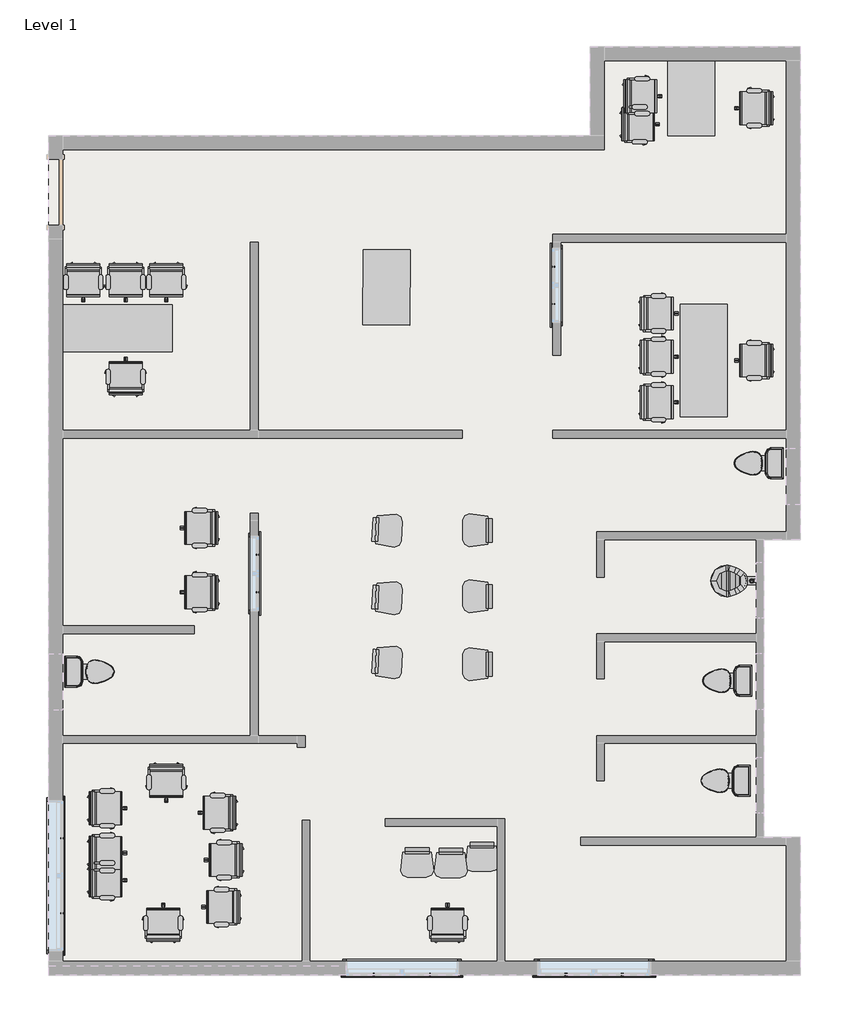
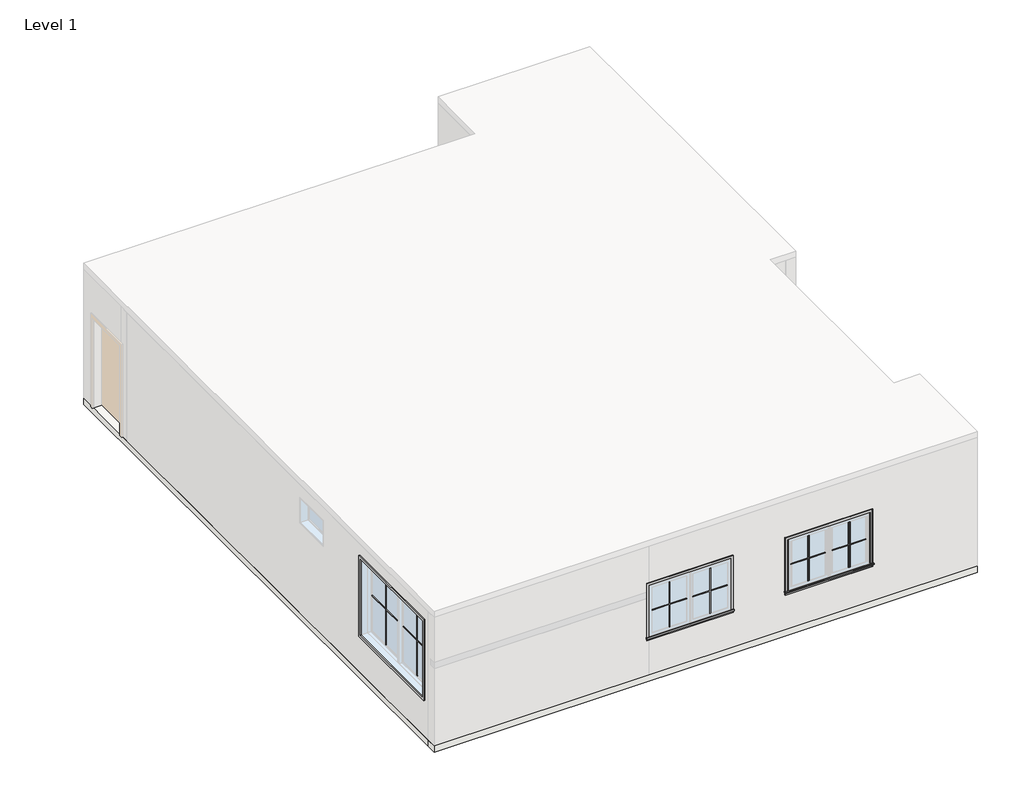
# One storey, part 2 of 2: 35 furniture elements, 28 proxies, 5 flow terminals, 2 slabs.
"""IFC4 building model written with IfcOpenShell, lengths in millimetres."""

from ifc_helpers import new_model, si_unit, frame, origin, place, context, project, spatial, polyline, outline, extrude, transform, mapped, element, save
from components import muntin_pattern_2x2_muntin_pattern_2x2_dc2504c2, muntin_pattern_2x2_muntin_pattern_2x2_0aa094e9, muntin_pattern_2x2_muntin_pattern_2x2_bb8d4d84, muntin_pattern_2x2_muntin_pattern_2x2_d03a1f3c, muntin_pattern_2x2_muntin_pattern_2x2_2b4d9f72, muntin_pattern_2x2_muntin_pattern_2x2_ef995ed3, trim_window_exterior_flat_with_sill_db7a9870, trim_window_exterior_flat_with_sill_02d88a07, trim_window_exterior_flat_with_sill_359ed2ce, trim_window_exterior_flat_with_sill_b7e4d11c, trim_window_interior_flat_picture_frame_bbff334a, trim_window_interior_flat_picture_frame_03e64d7c, trim_window_interior_flat_picture_frame_939a8053, trim_window_interior_flat_picture_frame_936b8d2a, flow_terminal_a02a0911, toilet_domestic_3d_toilet_domestic_3d_ba6479b0, toilet_domestic_3d_toilet_domestic_3d_30431060, chair_desk_chair_desk_7ad88740, chair_task_arms_chair_task_arms_bb362225, chair_task_arms_chair_task_arms_83a3c27c, furniture_acc2807d, furniture_03292632, furniture_fc20a73e, furniture_102a29e2

model = new_model("IFC4")

# Units and contexts
model_context = context("Model", 3, world=origin())
ifc_project = project(units=[si_unit("LENGTHUNIT", "METRE", prefix="MILLI")], contexts=[model_context])

# Site, building, storey
site = spatial("IfcSite", under=ifc_project)
building = spatial("IfcBuilding", under=site)
storey = spatial("IfcBuildingStorey", under=building, Name="Level 1", Elevation=0.0)

# Proxies
placement = place(None, origin())
muntin_pattern_2x2_muntin_pattern_2x2_shape = muntin_pattern_2x2_muntin_pattern_2x2_dc2504c2(model_context)
element("IfcBuildingElementProxy", 1, Name="Muntin Pattern_2x2 : Muntin Pattern_2x2", ObjectType="Muntin Pattern_2x2 : Muntin Pattern_2x2", at=placement, inside=storey, context=model_context, shape_type="MappedRepresentation", body=[
    mapped(muntin_pattern_2x2_muntin_pattern_2x2_shape, transform((-1125.8570713, -5476.875, 984.25), x_axis=(-1.0, 0.0, 0.0), y_axis=(0.0, -1.0, 0.0), z_axis=(0.0, 0.0, 1.0))),
])
element("IfcBuildingElementProxy", 2, Name="Muntin Pattern_2x2 : Muntin Pattern_2x2", ObjectType="Muntin Pattern_2x2 : Muntin Pattern_2x2", at=placement, inside=storey, context=model_context, shape_type="MappedRepresentation", body=[
    mapped(muntin_pattern_2x2_muntin_pattern_2x2_shape, transform((1979.6125, -5476.875, 984.25), x_axis=(-1.0, 0.0, 0.0), y_axis=(0.0, -1.0, 0.0), z_axis=(0.0, 0.0, 1.0))),
])
element("IfcBuildingElementProxy", 3, Name="Muntin Pattern_2x2 : Muntin Pattern_2x2", ObjectType="Muntin Pattern_2x2 : Muntin Pattern_2x2", at=placement, inside=storey, context=model_context, shape_type="MappedRepresentation", body=[
    mapped(muntin_pattern_2x2_muntin_pattern_2x2_shape, transform((2005.0125, -5476.875, 984.25), x_axis=(-1.0, 0.0, 0.0), y_axis=(0.0, -1.0, 0.0), z_axis=(0.0, 0.0, 1.0))),
])
muntin_pattern_2x2_muntin_pattern_2x2_2_shape = muntin_pattern_2x2_muntin_pattern_2x2_0aa094e9(model_context)
element("IfcBuildingElementProxy", 4, Name="Muntin Pattern_2x2 : Muntin Pattern_2x2", ObjectType="Muntin Pattern_2x2 : Muntin Pattern_2x2", at=placement, inside=storey, context=model_context, shape_type="MappedRepresentation", body=[
    mapped(muntin_pattern_2x2_muntin_pattern_2x2_2_shape, transform((-2037.0820713, -5476.875, 984.25), x_axis=(1.0, 0.0, 0.0), y_axis=(0.0, 1.0, 0.0), z_axis=(0.0, 0.0, 1.0))),
])
element("IfcBuildingElementProxy", 5, Name="Muntin Pattern_2x2 : Muntin Pattern_2x2", ObjectType="Muntin Pattern_2x2 : Muntin Pattern_2x2", at=placement, inside=storey, context=model_context, shape_type="MappedRepresentation", body=[
    mapped(muntin_pattern_2x2_muntin_pattern_2x2_2_shape, transform((1068.3875, -5476.875, 984.25), x_axis=(1.0, 0.0, 0.0), y_axis=(0.0, 1.0, 0.0), z_axis=(0.0, 0.0, 1.0))),
])
element("IfcBuildingElementProxy", 6, Name="Muntin Pattern_2x2 : Muntin Pattern_2x2", ObjectType="Muntin Pattern_2x2 : Muntin Pattern_2x2", at=placement, inside=storey, context=model_context, shape_type="MappedRepresentation", body=[
    mapped(muntin_pattern_2x2_muntin_pattern_2x2_2_shape, transform((1093.7875, -5476.875, 984.25), x_axis=(1.0, 0.0, 0.0), y_axis=(0.0, 1.0, 0.0), z_axis=(0.0, 0.0, 1.0))),
])
muntin_pattern_2x2_muntin_pattern_2x2_3_shape = muntin_pattern_2x2_muntin_pattern_2x2_bb8d4d84(model_context)
element("IfcBuildingElementProxy", 7, Name="Muntin Pattern_2x2 : Muntin Pattern_2x2", ObjectType="Muntin Pattern_2x2 : Muntin Pattern_2x2", at=placement, inside=storey, context=model_context, shape_type="MappedRepresentation", body=[
    mapped(muntin_pattern_2x2_muntin_pattern_2x2_3_shape, transform((-7096.125, -3265.4875, 984.25), x_axis=(0.0, -1.0, 0.0), y_axis=(1.0, 0.0, 0.0), z_axis=(0.0, 0.0, 1.0))),
])
muntin_pattern_2x2_muntin_pattern_2x2_4_shape = muntin_pattern_2x2_muntin_pattern_2x2_d03a1f3c(model_context)
element("IfcBuildingElementProxy", 8, Name="Muntin Pattern_2x2 : Muntin Pattern_2x2", ObjectType="Muntin Pattern_2x2 : Muntin Pattern_2x2", at=placement, inside=storey, context=model_context, shape_type="MappedRepresentation", body=[
    mapped(muntin_pattern_2x2_muntin_pattern_2x2_4_shape, transform((-7096.125, -4481.5125, 984.25), x_axis=(0.0, 1.0, 0.0), y_axis=(-1.0, 0.0, 0.0), z_axis=(0.0, 0.0, 1.0))),
])
muntin_pattern_2x2_muntin_pattern_2x2_5_shape = muntin_pattern_2x2_muntin_pattern_2x2_2b4d9f72(model_context)
element("IfcBuildingElementProxy", 9, Name="Muntin Pattern_2x2 : Muntin Pattern_2x2", ObjectType="Muntin Pattern_2x2 : Muntin Pattern_2x2", at=placement, inside=storey, context=model_context, shape_type="MappedRepresentation", body=[
    mapped(muntin_pattern_2x2_muntin_pattern_2x2_5_shape, transform((-3921.125, 1332.4236463, 984.25), x_axis=(0.0, -1.0, 0.0), y_axis=(1.0, 0.0, 0.0), z_axis=(0.0, 0.0, 1.0))),
])
element("IfcBuildingElementProxy", 10, Name="Muntin Pattern_2x2 : Muntin Pattern_2x2", ObjectType="Muntin Pattern_2x2 : Muntin Pattern_2x2", at=placement, inside=storey, context=model_context, shape_type="MappedRepresentation", body=[
    mapped(muntin_pattern_2x2_muntin_pattern_2x2_5_shape, transform((-3921.125, 1332.4236463, 984.25), x_axis=(0.0, -1.0, 0.0), y_axis=(1.0, 0.0, 0.0), z_axis=(0.0, 0.0, 1.0))),
])
element("IfcBuildingElementProxy", 11, Name="Muntin Pattern_2x2 : Muntin Pattern_2x2", ObjectType="Muntin Pattern_2x2 : Muntin Pattern_2x2", at=placement, inside=storey, context=model_context, shape_type="MappedRepresentation", body=[
    mapped(muntin_pattern_2x2_muntin_pattern_2x2_5_shape, transform((873.125, 5399.0875, 984.25), x_axis=(0.0, 1.0, 0.0), y_axis=(-1.0, 0.0, 0.0), z_axis=(0.0, 0.0, 1.0))),
])
muntin_pattern_2x2_muntin_pattern_2x2_6_shape = muntin_pattern_2x2_muntin_pattern_2x2_ef995ed3(model_context)
element("IfcBuildingElementProxy", 12, Name="Muntin Pattern_2x2 : Muntin Pattern_2x2", ObjectType="Muntin Pattern_2x2 : Muntin Pattern_2x2", at=placement, inside=storey, context=model_context, shape_type="MappedRepresentation", body=[
    mapped(muntin_pattern_2x2_muntin_pattern_2x2_6_shape, transform((-3921.125, 725.9986463, 984.25), x_axis=(0.0, 1.0, 0.0), y_axis=(-1.0, 0.0, 0.0), z_axis=(0.0, 0.0, 1.0))),
])
element("IfcBuildingElementProxy", 13, Name="Muntin Pattern_2x2 : Muntin Pattern_2x2", ObjectType="Muntin Pattern_2x2 : Muntin Pattern_2x2", at=placement, inside=storey, context=model_context, shape_type="MappedRepresentation", body=[
    mapped(muntin_pattern_2x2_muntin_pattern_2x2_6_shape, transform((-3921.125, 725.9986463, 984.25), x_axis=(0.0, 1.0, 0.0), y_axis=(-1.0, 0.0, 0.0), z_axis=(0.0, 0.0, 1.0))),
])
element("IfcBuildingElementProxy", 14, Name="Muntin Pattern_2x2 : Muntin Pattern_2x2", ObjectType="Muntin Pattern_2x2 : Muntin Pattern_2x2", at=placement, inside=storey, context=model_context, shape_type="MappedRepresentation", body=[
    mapped(muntin_pattern_2x2_muntin_pattern_2x2_6_shape, transform((873.125, 6005.5125, 984.25), x_axis=(0.0, -1.0, 0.0), y_axis=(1.0, 0.0, 0.0), z_axis=(0.0, 0.0, 1.0))),
])
trim_window_exterior_flat_with_sill_shape = trim_window_exterior_flat_with_sill_db7a9870(model_context)
element("IfcBuildingElementProxy", 15, Name="Trim-Window-Exterior-Flat : with Sill", ObjectType="Trim-Window-Exterior-Flat : with Sill", at=placement, inside=storey, context=model_context, shape_type="MappedRepresentation", body=[
    mapped(trim_window_exterior_flat_with_sill_shape, transform((-1581.4695713, -5486.4, 2133.6), x_axis=(-1.0, 0.0, 0.0), y_axis=(0.0, 0.0, -1.0), z_axis=(0.0, -1.0, 0.0))),
])
trim_window_exterior_flat_with_sill_2_shape = trim_window_exterior_flat_with_sill_02d88a07(model_context)
element("IfcBuildingElementProxy", 16, Name="Trim-Window-Exterior-Flat : with Sill", ObjectType="Trim-Window-Exterior-Flat : with Sill", at=placement, inside=storey, context=model_context, shape_type="MappedRepresentation", body=[
    mapped(trim_window_exterior_flat_with_sill_2_shape, transform((1524.0, -5486.4, 2133.6), x_axis=(1.0, 0.0, 0.0), y_axis=(0.0, 0.0, 1.0), z_axis=(0.0, -1.0, 0.0))),
])
element("IfcBuildingElementProxy", 17, Name="Trim-Window-Exterior-Flat : with Sill", ObjectType="Trim-Window-Exterior-Flat : with Sill", at=placement, inside=storey, context=model_context, shape_type="MappedRepresentation", body=[
    mapped(trim_window_exterior_flat_with_sill_2_shape, transform((1549.4, -5486.4, 2133.6), x_axis=(1.0, 0.0, 0.0), y_axis=(0.0, 0.0, 1.0), z_axis=(0.0, -1.0, 0.0))),
])
trim_window_exterior_flat_with_sill_3_shape = trim_window_exterior_flat_with_sill_359ed2ce(model_context)
element("IfcBuildingElementProxy", 18, Name="Trim-Window-Exterior-Flat : with Sill", ObjectType="Trim-Window-Exterior-Flat : with Sill", at=placement, inside=storey, context=model_context, shape_type="MappedRepresentation", body=[
    mapped(trim_window_exterior_flat_with_sill_3_shape, transform((-7086.6, -3873.5, 2743.2), x_axis=(0.0, 1.0, 0.0), y_axis=(0.0, 0.0, 1.0), z_axis=(1.0, 0.0, 0.0))),
])
trim_window_exterior_flat_with_sill_4_shape = trim_window_exterior_flat_with_sill_b7e4d11c(model_context)
element("IfcBuildingElementProxy", 19, Name="Trim-Window-Exterior-Flat : with Sill", ObjectType="Trim-Window-Exterior-Flat : with Sill", at=placement, inside=storey, context=model_context, shape_type="MappedRepresentation", body=[
    mapped(trim_window_exterior_flat_with_sill_4_shape, transform((-3911.6, 1029.2111463, 2743.2), x_axis=(0.0, 1.0, 0.0), y_axis=(0.0, 0.0, 1.0), z_axis=(1.0, 0.0, 0.0))),
])
element("IfcBuildingElementProxy", 20, Name="Trim-Window-Exterior-Flat : with Sill", ObjectType="Trim-Window-Exterior-Flat : with Sill", at=placement, inside=storey, context=model_context, shape_type="MappedRepresentation", body=[
    mapped(trim_window_exterior_flat_with_sill_4_shape, transform((-3911.6, 1029.2111463, 2743.2), x_axis=(0.0, 1.0, 0.0), y_axis=(0.0, 0.0, 1.0), z_axis=(1.0, 0.0, 0.0))),
])
element("IfcBuildingElementProxy", 21, Name="Trim-Window-Exterior-Flat : with Sill", ObjectType="Trim-Window-Exterior-Flat : with Sill", at=placement, inside=storey, context=model_context, shape_type="MappedRepresentation", body=[
    mapped(trim_window_exterior_flat_with_sill_4_shape, transform((863.6, 5702.3, 2743.2), x_axis=(0.0, -1.0, 0.0), y_axis=(0.0, 0.0, 1.0), z_axis=(-1.0, 0.0, 0.0))),
])
trim_window_interior_flat_picture_frame_shape = trim_window_interior_flat_picture_frame_bbff334a(model_context)
element("IfcBuildingElementProxy", 22, Name="Trim-Window-Interior-Flat : Picture Frame", ObjectType="Trim-Window-Interior-Flat : Picture Frame", at=placement, inside=storey, context=model_context, shape_type="MappedRepresentation", body=[
    mapped(trim_window_interior_flat_picture_frame_shape, transform((-1581.4695713, -5257.8, 2133.6), x_axis=(1.0, 0.0, 0.0), y_axis=(0.0, 0.0, -1.0), z_axis=(0.0, 1.0, 0.0))),
])
trim_window_interior_flat_picture_frame_2_shape = trim_window_interior_flat_picture_frame_03e64d7c(model_context)
element("IfcBuildingElementProxy", 23, Name="Trim-Window-Interior-Flat : Picture Frame", ObjectType="Trim-Window-Interior-Flat : Picture Frame", at=placement, inside=storey, context=model_context, shape_type="MappedRepresentation", body=[
    mapped(trim_window_interior_flat_picture_frame_2_shape, transform((1524.0, -5257.8, 2133.6), x_axis=(-1.0, 0.0, 0.0), y_axis=(0.0, 0.0, 1.0), z_axis=(0.0, 1.0, 0.0))),
])
element("IfcBuildingElementProxy", 24, Name="Trim-Window-Interior-Flat : Picture Frame", ObjectType="Trim-Window-Interior-Flat : Picture Frame", at=placement, inside=storey, context=model_context, shape_type="MappedRepresentation", body=[
    mapped(trim_window_interior_flat_picture_frame_2_shape, transform((1549.4, -5257.8, 2133.6), x_axis=(-1.0, 0.0, 0.0), y_axis=(0.0, 0.0, 1.0), z_axis=(0.0, 1.0, 0.0))),
])
trim_window_interior_flat_picture_frame_3_shape = trim_window_interior_flat_picture_frame_939a8053(model_context)
element("IfcBuildingElementProxy", 25, Name="Trim-Window-Interior-Flat : Picture Frame", ObjectType="Trim-Window-Interior-Flat : Picture Frame", at=placement, inside=storey, context=model_context, shape_type="MappedRepresentation", body=[
    mapped(trim_window_interior_flat_picture_frame_3_shape, transform((-7315.2, -3873.5, 2743.2), x_axis=(0.0, -1.0, 0.0), y_axis=(0.0, 0.0, 1.0), z_axis=(-1.0, 0.0, 0.0))),
])
trim_window_interior_flat_picture_frame_4_shape = trim_window_interior_flat_picture_frame_936b8d2a(model_context)
element("IfcBuildingElementProxy", 26, Name="Trim-Window-Interior-Flat : Picture Frame", ObjectType="Trim-Window-Interior-Flat : Picture Frame", at=placement, inside=storey, context=model_context, shape_type="MappedRepresentation", body=[
    mapped(trim_window_interior_flat_picture_frame_4_shape, transform((-4038.6, 1029.2111463, 2743.2), x_axis=(0.0, -1.0, 0.0), y_axis=(0.0, 0.0, 1.0), z_axis=(-1.0, 0.0, 0.0))),
])
element("IfcBuildingElementProxy", 27, Name="Trim-Window-Interior-Flat : Picture Frame", ObjectType="Trim-Window-Interior-Flat : Picture Frame", at=placement, inside=storey, context=model_context, shape_type="MappedRepresentation", body=[
    mapped(trim_window_interior_flat_picture_frame_4_shape, transform((-4038.6, 1029.2111463, 2743.2), x_axis=(0.0, -1.0, 0.0), y_axis=(0.0, 0.0, 1.0), z_axis=(-1.0, 0.0, 0.0))),
])
element("IfcBuildingElementProxy", 28, Name="Trim-Window-Interior-Flat : Picture Frame", ObjectType="Trim-Window-Interior-Flat : Picture Frame", at=placement, inside=storey, context=model_context, shape_type="MappedRepresentation", body=[
    mapped(trim_window_interior_flat_picture_frame_4_shape, transform((990.6, 5702.3, 2743.2), x_axis=(0.0, 1.0, 0.0), y_axis=(0.0, 0.0, 1.0), z_axis=(1.0, 0.0, 0.0))),
])

# Flow terminals
flow_terminal_shape = flow_terminal_a02a0911(model_context)
element("IfcFlowTerminal", 29, ObjectType="Toilet-Commercial-Wall-3D : 15\" Seat Height", at=placement, inside=storey, context=model_context, shape_type="MappedRepresentation", body=[
    mapped(flow_terminal_shape, transform((4225.925, 503.8174373, 0.0), x_axis=(0.0, 1.0, 0.0), y_axis=(-1.0, 0.0, 0.0), z_axis=(0.0, 0.0, 1.0))),
])
toilet_domestic_3d_toilet_domestic_3d_shape = toilet_domestic_3d_toilet_domestic_3d_ba6479b0(model_context)
toilet_domestic_3d_toilet_domestic_3d_2_shape = toilet_domestic_3d_toilet_domestic_3d_30431060(model_context)
element("IfcFlowTerminal", 30, ObjectType="Toilet-Domestic-3D : Toilet-Domestic-3D", at=placement, inside=storey, context=model_context, shape_type="MappedRepresentation", body=[
    mapped(toilet_domestic_3d_toilet_domestic_3d_shape, transform((3600.5018648, -710.8948966, 0.0), x_axis=(0.0, -1.0, 0.0), y_axis=(1.0, 0.0, 0.0), z_axis=(0.0, 0.0, 1.0))),
    mapped(toilet_domestic_3d_toilet_domestic_3d_2_shape, transform((3600.5018648, -710.8948966, 0.0), x_axis=(0.0, -1.0, 0.0), y_axis=(1.0, 0.0, 0.0), z_axis=(0.0, 0.0, 1.0))),
])
element("IfcFlowTerminal", 31, ObjectType="Toilet-Domestic-3D : Toilet-Domestic-3D", at=placement, inside=storey, context=model_context, shape_type="MappedRepresentation", body=[
    mapped(toilet_domestic_3d_toilet_domestic_3d_shape, transform((3574.6912015, -2333.2020056, 0.0), x_axis=(0.0, -1.0, 0.0), y_axis=(1.0, 0.0, 0.0), z_axis=(0.0, 0.0, 1.0))),
    mapped(toilet_domestic_3d_toilet_domestic_3d_2_shape, transform((3574.6912015, -2333.2020056, 0.0), x_axis=(0.0, -1.0, 0.0), y_axis=(1.0, 0.0, 0.0), z_axis=(0.0, 0.0, 1.0))),
])
element("IfcFlowTerminal", 32, ObjectType="Toilet-Domestic-3D : Toilet-Domestic-3D", at=placement, inside=storey, context=model_context, shape_type="MappedRepresentation", body=[
    mapped(toilet_domestic_3d_toilet_domestic_3d_shape, transform((-6555.3800667, -564.8480137, 0.0), x_axis=(0.0, 1.0, 0.0), y_axis=(-1.0, 0.0, 0.0), z_axis=(0.0, 0.0, 1.0))),
    mapped(toilet_domestic_3d_toilet_domestic_3d_2_shape, transform((-6555.3800667, -564.8480137, 0.0), x_axis=(0.0, 1.0, 0.0), y_axis=(-1.0, 0.0, 0.0), z_axis=(0.0, 0.0, 1.0))),
])
element("IfcFlowTerminal", 33, ObjectType="Toilet-Domestic-3D : Toilet-Domestic-3D", at=placement, inside=storey, context=model_context, shape_type="MappedRepresentation", body=[
    mapped(toilet_domestic_3d_toilet_domestic_3d_shape, transform((4111.625, 2817.0462711, 0.0), x_axis=(0.0, -1.0, 0.0), y_axis=(1.0, 0.0, 0.0), z_axis=(0.0, 0.0, 1.0))),
    mapped(toilet_domestic_3d_toilet_domestic_3d_2_shape, transform((4111.625, 2817.0462711, 0.0), x_axis=(0.0, -1.0, 0.0), y_axis=(1.0, 0.0, 0.0), z_axis=(0.0, 0.0, 1.0))),
])

# Furniture
chair_desk_chair_desk_shape = chair_desk_chair_desk_7ad88740(model_context)
element("IfcFurniture", 34, ObjectType="Chair-Desk : Chair-Desk", at=placement, inside=storey, context=model_context, shape_type="MappedRepresentation", body=[
    mapped(chair_desk_chair_desk_shape, transform((-186.696437, 1729.5851392, 0.0), x_axis=(0.0, 1.0, 0.0), y_axis=(-1.0, 0.0, 0.0), z_axis=(0.0, 0.0, 1.0))),
])
element("IfcFurniture", 35, ObjectType="Chair-Desk : Chair-Desk", at=placement, inside=storey, context=model_context, shape_type="MappedRepresentation", body=[
    mapped(chair_desk_chair_desk_shape, transform((-186.696437, 659.318602, 0.0), x_axis=(0.0, 1.0, 0.0), y_axis=(-1.0, 0.0, 0.0), z_axis=(0.0, 0.0, 1.0))),
])
element("IfcFurniture", 36, ObjectType="Chair-Desk : Chair-Desk", at=placement, inside=storey, context=model_context, shape_type="MappedRepresentation", body=[
    mapped(chair_desk_chair_desk_shape, transform((-186.696437, -441.6562876, 0.0), x_axis=(0.0, 1.0, 0.0), y_axis=(-1.0, 0.0, 0.0), z_axis=(0.0, 0.0, 1.0))),
])
element("IfcFurniture", 37, ObjectType="Chair-Desk : Chair-Desk", at=placement, inside=storey, context=model_context, shape_type="MappedRepresentation", body=[
    mapped(chair_desk_chair_desk_shape, transform((-1992.3517418, 1738.144391, 0.0), x_axis=(-0.051641684914146245, -0.9986656779819902, 0.0), y_axis=(0.9986656779819902, -0.051641684914146245, 0.0), z_axis=(0.0, 0.0, 1.0))),
])
element("IfcFurniture", 38, ObjectType="Chair-Desk : Chair-Desk", at=placement, inside=storey, context=model_context, shape_type="MappedRepresentation", body=[
    mapped(chair_desk_chair_desk_shape, transform((-1992.3517418, 640.8125907, 0.0), x_axis=(-0.051641684914146245, -0.9986656779819902, 0.0), y_axis=(0.9986656779819902, -0.051641684914146245, 0.0), z_axis=(0.0, 0.0, 1.0))),
])
element("IfcFurniture", 39, ObjectType="Chair-Desk : Chair-Desk", at=placement, inside=storey, context=model_context, shape_type="MappedRepresentation", body=[
    mapped(chair_desk_chair_desk_shape, transform((-1992.3517418, -400.5874093, 0.0), x_axis=(-0.051641684914146245, -0.9986656779819902, 0.0), y_axis=(0.9986656779819902, -0.051641684914146245, 0.0), z_axis=(0.0, 0.0, 1.0))),
])
element("IfcFurniture", 40, ObjectType="Chair-Desk : Chair-Desk", at=placement, inside=storey, context=model_context, shape_type="MappedRepresentation", body=[
    mapped(chair_desk_chair_desk_shape, transform((-1336.2779178, -3490.3358848, 0.0), x_axis=(-1.0, 0.0, 0.0), y_axis=(0.0, -1.0, 0.0), z_axis=(0.0, 0.0, 1.0))),
])
element("IfcFurniture", 41, ObjectType="Chair-Desk : Chair-Desk", at=placement, inside=storey, context=model_context, shape_type="MappedRepresentation", body=[
    mapped(chair_desk_chair_desk_shape, transform((-788.0882588, -3498.2498137, 0.0), x_axis=(-1.0, 0.0, 0.0), y_axis=(0.0, -1.0, 0.0), z_axis=(0.0, 0.0, 1.0))),
])
element("IfcFurniture", 42, ObjectType="Chair-Desk : Chair-Desk", at=placement, inside=storey, context=model_context, shape_type="MappedRepresentation", body=[
    mapped(chair_desk_chair_desk_shape, transform((-283.9315487, -3398.845913, 0.0), x_axis=(-1.0, 0.0, 0.0), y_axis=(0.0, -1.0, 0.0), z_axis=(0.0, 0.0, 1.0))),
])
chair_task_arms_chair_task_arms_shape = chair_task_arms_chair_task_arms_bb362225(model_context)
element("IfcFurniture", 43, ObjectType="Chair-Task Arms : Chair-Task Arms", at=placement, inside=storey, context=model_context, shape_type="MappedRepresentation", body=[
    mapped(chair_task_arms_chair_task_arms_shape, transform((2533.7540984, 5386.0908197, 0.0), x_axis=(0.0, -1.0, 0.0), y_axis=(1.0, 0.0, 0.0), z_axis=(0.0, 0.0, 1.0))),
])
element("IfcFurniture", 44, ObjectType="Chair-Task Arms : Chair-Task Arms", at=placement, inside=storey, context=model_context, shape_type="MappedRepresentation", body=[
    mapped(chair_task_arms_chair_task_arms_shape, transform((2533.7540984, 3945.6565809, 0.0), x_axis=(0.0, -1.0, 0.0), y_axis=(1.0, 0.0, 0.0), z_axis=(0.0, 0.0, 1.0))),
])
element("IfcFurniture", 45, ObjectType="Chair-Task Arms : Chair-Task Arms", at=placement, inside=storey, context=model_context, shape_type="MappedRepresentation", body=[
    mapped(chair_task_arms_chair_task_arms_shape, transform((2533.7540984, 4686.9202237, 0.0), x_axis=(0.0, -1.0, 0.0), y_axis=(1.0, 0.0, 0.0), z_axis=(0.0, 0.0, 1.0))),
])
element("IfcFurniture", 46, ObjectType="Chair-Task Arms : Chair-Task Arms", at=placement, inside=storey, context=model_context, shape_type="MappedRepresentation", body=[
    mapped(chair_task_arms_chair_task_arms_shape, transform((4181.3709016, 4342.1091803, 0.0), x_axis=(0.0, 1.0, 0.0), y_axis=(-1.0, 0.0, 0.0), z_axis=(0.0, 0.0, 1.0))),
])
element("IfcFurniture", 47, ObjectType="Chair-Task Arms : Chair-Task Arms", at=placement, inside=storey, context=model_context, shape_type="MappedRepresentation", body=[
    mapped(chair_task_arms_chair_task_arms_shape, transform((-6609.2997508, 5802.6774893, 0.0), x_axis=(-1.0, 0.0, 0.0), y_axis=(0.0, -1.0, 0.0), z_axis=(0.0, 0.0, 1.0))),
])
element("IfcFurniture", 48, ObjectType="Chair-Task Arms : Chair-Task Arms", at=placement, inside=storey, context=model_context, shape_type="MappedRepresentation", body=[
    mapped(chair_task_arms_chair_task_arms_shape, transform((-5923.4997508, 5802.6774893, 0.0), x_axis=(-1.0, 0.0, 0.0), y_axis=(0.0, -1.0, 0.0), z_axis=(0.0, 0.0, 1.0))),
])
element("IfcFurniture", 49, ObjectType="Chair-Task Arms : Chair-Task Arms", at=placement, inside=storey, context=model_context, shape_type="MappedRepresentation", body=[
    mapped(chair_task_arms_chair_task_arms_shape, transform((-5263.0997508, 5802.6774893, 0.0), x_axis=(-1.0, 0.0, 0.0), y_axis=(0.0, -1.0, 0.0), z_axis=(0.0, 0.0, 1.0))),
])
element("IfcFurniture", 50, ObjectType="Chair-Task Arms : Chair-Task Arms", at=placement, inside=storey, context=model_context, shape_type="MappedRepresentation", body=[
    mapped(chair_task_arms_chair_task_arms_shape, transform((4181.3709016, 8435.9379864, 0.0), x_axis=(0.0, 1.0, 0.0), y_axis=(-1.0, 0.0, 0.0), z_axis=(0.0, 0.0, 1.0))),
])
element("IfcFurniture", 51, ObjectType="Chair-Task Arms : Chair-Task Arms", at=placement, inside=storey, context=model_context, shape_type="MappedRepresentation", body=[
    mapped(chair_task_arms_chair_task_arms_shape, transform((2267.0540984, 8911.4381912, 0.0), x_axis=(0.0, -1.0, 0.0), y_axis=(1.0, 0.0, 0.0), z_axis=(0.0, 0.0, 1.0))),
])
element("IfcFurniture", 52, ObjectType="Chair-Task Arms : Chair-Task Arms", at=placement, inside=storey, context=model_context, shape_type="MappedRepresentation", body=[
    mapped(chair_task_arms_chair_task_arms_shape, transform((2228.9540984, 8454.2381912, 0.0), x_axis=(0.0, -1.0, 0.0), y_axis=(1.0, 0.0, 0.0), z_axis=(0.0, 0.0, 1.0))),
])
element("IfcFurniture", 53, ObjectType="Chair-Task Arms : Chair-Task Arms", at=placement, inside=storey, context=model_context, shape_type="MappedRepresentation", body=[
    mapped(chair_task_arms_chair_task_arms_shape, transform((-4817.0756514, 1625.3539409, 0.0), x_axis=(0.0, 1.0, 0.0), y_axis=(-1.0, 0.0, 0.0), z_axis=(0.0, 0.0, 1.0))),
])
element("IfcFurniture", 54, ObjectType="Chair-Task Arms : Chair-Task Arms", at=placement, inside=storey, context=model_context, shape_type="MappedRepresentation", body=[
    mapped(chair_task_arms_chair_task_arms_shape, transform((-4817.0756514, 583.3573936, 0.0), x_axis=(0.0, 1.0, 0.0), y_axis=(-1.0, 0.0, 0.0), z_axis=(0.0, 0.0, 1.0))),
])
element("IfcFurniture", 55, ObjectType="Chair-Task Arms : Chair-Task Arms", at=placement, inside=storey, context=model_context, shape_type="MappedRepresentation", body=[
    mapped(chair_task_arms_chair_task_arms_shape, transform((-4522.4685104, -2995.6992242, 0.0), x_axis=(0.0, 1.0, 0.0), y_axis=(-1.0, 0.0, 0.0), z_axis=(0.0, 0.0, 1.0))),
])
element("IfcFurniture", 56, ObjectType="Chair-Task Arms : Chair-Task Arms", at=placement, inside=storey, context=model_context, shape_type="MappedRepresentation", body=[
    mapped(chair_task_arms_chair_task_arms_shape, transform((-4420.2882293, -3759.9572054, 0.0), x_axis=(0.0, 1.0, 0.0), y_axis=(-1.0, 0.0, 0.0), z_axis=(0.0, 0.0, 1.0))),
])
element("IfcFurniture", 57, ObjectType="Chair-Task Arms : Chair-Task Arms", at=placement, inside=storey, context=model_context, shape_type="MappedRepresentation", body=[
    mapped(chair_task_arms_chair_task_arms_shape, transform((-4461.677653, -4522.3529931, 0.0), x_axis=(0.0, 1.0, 0.0), y_axis=(-1.0, 0.0, 0.0), z_axis=(0.0, 0.0, 1.0))),
])
element("IfcFurniture", 58, ObjectType="Chair-Task Arms : Chair-Task Arms", at=placement, inside=storey, context=model_context, shape_type="MappedRepresentation", body=[
    mapped(chair_task_arms_chair_task_arms_shape, transform((-6410.1861871, -2639.8091917, 0.0), x_axis=(0.0, -1.0, 0.0), y_axis=(1.0, 0.0, 0.0), z_axis=(0.0, 0.0, 1.0))),
])
element("IfcFurniture", 59, ObjectType="Chair-Task Arms : Chair-Task Arms", at=placement, inside=storey, context=model_context, shape_type="MappedRepresentation", body=[
    mapped(chair_task_arms_chair_task_arms_shape, transform((-6410.1861871, -3363.7091917, 0.0), x_axis=(0.0, -1.0, 0.0), y_axis=(1.0, 0.0, 0.0), z_axis=(0.0, 0.0, 1.0))),
])
element("IfcFurniture", 60, ObjectType="Chair-Task Arms : Chair-Task Arms", at=placement, inside=storey, context=model_context, shape_type="MappedRepresentation", body=[
    mapped(chair_task_arms_chair_task_arms_shape, transform((-6410.1861871, -3808.4533853, 0.0), x_axis=(0.0, -1.0, 0.0), y_axis=(1.0, 0.0, 0.0), z_axis=(0.0, 0.0, 1.0))),
])
element("IfcFurniture", 61, ObjectType="Chair-Task Arms : Chair-Task Arms", at=placement, inside=storey, context=model_context, shape_type="MappedRepresentation", body=[
    mapped(chair_task_arms_chair_task_arms_shape, transform((-5263.0997508, -2314.256104, 0.0), x_axis=(-1.0, 0.0, 0.0), y_axis=(0.0, -1.0, 0.0), z_axis=(0.0, 0.0, 1.0))),
])
chair_task_arms_chair_task_arms_2_shape = chair_task_arms_chair_task_arms_83a3c27c(model_context)
element("IfcFurniture", 62, ObjectType="Chair-Task Arms : Chair-Task Arms", at=placement, inside=storey, context=model_context, shape_type="MappedRepresentation", body=[
    mapped(chair_task_arms_chair_task_arms_2_shape, transform((-5923.4997508, 4175.200127, 0.0), x_axis=(-1.0, 0.0, 0.0), y_axis=(0.0, -1.0, 0.0), z_axis=(0.0, 0.0, 1.0))),
])
element("IfcFurniture", 63, ObjectType="Chair-Task Arms : Chair-Task Arms", at=placement, inside=storey, context=model_context, shape_type="MappedRepresentation", body=[
    mapped(chair_task_arms_chair_task_arms_2_shape, transform((-5313.8997508, -4688.3141044, 0.0), x_axis=(-1.0, 0.0, 0.0), y_axis=(0.0, -1.0, 0.0), z_axis=(0.0, 0.0, 1.0))),
])
element("IfcFurniture", 64, ObjectType="Chair-Task Arms : Chair-Task Arms", at=placement, inside=storey, context=model_context, shape_type="MappedRepresentation", body=[
    mapped(chair_task_arms_chair_task_arms_2_shape, transform((-701.1834758, -4688.3141044, 0.0), x_axis=(-1.0, 0.0, 0.0), y_axis=(0.0, -1.0, 0.0), z_axis=(0.0, 0.0, 1.0))),
])
furniture_shape = furniture_acc2807d(model_context)
element("IfcFurniture", 65, ObjectType="Table-Coffee Rectangular : 48\" x 30\"", at=placement, inside=storey, context=model_context, shape_type="MappedRepresentation", body=[
    mapped(furniture_shape, transform((-1464.6406329, 5055.025631, 0.0), x_axis=(0.00443889505176337, 0.9999901480568293, 0.0), y_axis=(-0.9999901480568293, 0.00443889505176337, 0.0), z_axis=(0.0, 0.0, 1.0))),
])
furniture_2_shape = furniture_03292632(model_context)
element("IfcFurniture", 66, ObjectType="Table-Rectangular : 72\" x 30\"", at=placement, inside=storey, context=model_context, shape_type="MappedRepresentation", body=[
    mapped(furniture_2_shape, transform((3314.7, 4483.1, 0.0), x_axis=(0.0, 1.0, 0.0), y_axis=(-1.0, 0.0, 0.0), z_axis=(0.0, 0.0, 1.0))),
])
furniture_3_shape = furniture_fc20a73e(model_context)
element("IfcFurniture", 67, ObjectType="Table-Rectangular : 72\" x 30\" 2", at=placement, inside=storey, context=model_context, shape_type="MappedRepresentation", body=[
    mapped(furniture_3_shape, transform((3111.5, 8737.6, 0.0), x_axis=(0.0, 1.0, 0.0), y_axis=(-1.0, 0.0, 0.0), z_axis=(0.0, 0.0, 1.0))),
])
furniture_4_shape = furniture_102a29e2(model_context)
element("IfcFurniture", 68, ObjectType="Table-Rectangular : 72\" x 30\" 3", at=placement, inside=storey, context=model_context, shape_type="MappedRepresentation", body=[
    mapped(furniture_4_shape, transform((-6197.6, 5003.8, 0.0), x_axis=(1.0, 0.0, 0.0), y_axis=(0.0, 1.0, 0.0), z_axis=(0.0, 0.0, 1.0))),
])

# Slabs
element("IfcSlab", 69, ObjectType="Generic - 6\" 2", at=placement, inside=storey, context=model_context, shape_type="SweptSolid", body=[
    extrude(outline(polyline([(-7315.2, 8128.0), (1473.2, 8128.0), (1473.2, 9575.8), (4876.8, 9575.8), (4876.8, 1574.8), (4289.425, 1574.8), (4289.425, -3251.2), (4876.8, -3251.2), (4876.8, -5486.4), (-7315.2, -5486.4), (-7315.2, -5257.8), (-7315.2, 8128.0)])), frame((0.0, 0.0, -152.4), z_axis=(0.0, 0.0, 1.0), x_axis=(1.0, 0.0, 0.0)), (0.0, 0.0, 1.0), 152.4),
])
element("IfcSlab", 70, ObjectType="Generic - 6\" 2", at=placement, inside=storey, context=model_context, shape_type="SweptSolid", body=[
    extrude(outline(polyline([(-7315.2, -5257.8), (-7315.2, 8128.0), (1473.2, 8128.0), (1473.2, 9575.8), (4876.8, 9575.8), (4876.8, 1574.8), (4289.425, 1574.8), (4289.425, -3251.2), (4876.8, -3251.2), (4876.8, -5486.4), (-7315.2, -5486.4), (-7315.2, -5257.8)])), frame((0.0, 0.0, -152.4), z_axis=(0.0, 0.0, 1.0), x_axis=(1.0, 0.0, 0.0)), (0.0, 0.0, 1.0), 152.4),
])

save(model, "model.ifc")

# Revit data of these elements
# Type "Muntin Pattern_2x2 : Muntin Pattern_2x2"
#   Width [instance default] = 4' - 0"
#   Thickness = 0' - 0 1/2"
#   Height [instance default] = 4' - 0"
#   Distance = 0' - 0 3/4"
#   Interior Material [instance default] = none
#   Exterior Material [instance default] = none
#   Default Elevation = 0
# Type "Trim-Window-Exterior-Flat : with Sill"
#   Trim Width = 0' - 2 1/4"
#   Trim Thickness_Picture Frame = 0' - 1 1/4"
#   Trim Thickness_with Sill = 0' - 0 3/4"
#   Sill Thickness = 0' - 1 1/4"
#   Opening Width [instance default] = 2' - 0"
#   Opening Height [instance default] = 3' - 0"
#   Default Elevation = 4' - 0"
#   Sill = yes
#   Picture Frame = no
#   Trim Material [instance default] = none
# Type "Trim-Window-Interior-Flat : Picture Frame"
#   Trim Thickness_Picture Frame = 0' - 1 1/4"
#   Trim Width = 0' - 2 1/4"
#   Trim Thickness_with Sill = 0' - 0 3/4"
#   Sill Thickness = 0' - 1 1/4"
#   Opening Width [instance default] = 2' - 0"
#   Opening Height [instance default] = 3' - 0"
#   Default Elevation = 4' - 0"
#   Sill = no
#   Picture Frame = yes
#   Trim Material [instance default] = none
# Type "Toilet-Commercial-Wall-3D : 15\" Seat Height"
#   Assembly Code = "D2010110"
#   Mounting Height = 1' - 3"
#   Piping Material = Steel, Polished
#   Toilet - Bowl Material = Porcelain, Ivory
#   Toilet - Seat Material = Laminate, Ivory, Matte
#   Default Elevation = 0
# Type "Toilet-Domestic-3D : Toilet-Domestic-3D"
#   Assembly Code = "D2010110"
#   Toilet - Bowl/Basin Material = Porcelain, Linen
#   Toilet - Seat Material = Laminate, Linen, Matte
#   Default Elevation = 0
# Type "Chair-Desk : Chair-Desk"
#   Assembly Code = "E2020200"
#   Seat/Back Material = Textile - Slate Blue
#   Base Material = Steel, Chrome Plated
#   Default Elevation = 0
# Type "Chair-Task Arms : Chair-Task Arms"
#   Assembly Code = "E2020200"
#   Base Material = Plastic, Opaque Black
#   Caster Material = Plastic, Opaque Black
#   Seat/Back Material = Textile - Slate Blue
#   Default Elevation = 0
# Type "Table-Coffee Rectangular : 48\" x 30\""
#   Assembly Code = "E2020200"
#   Height = 1' - 1"
#   Length = 4' - 0"
#   Width = 2' - 6"
#   Base Material = Metal - Chrome
#   Table Top Material = Glass - Clear, Grey
#   Default Elevation = 0
# Type "Table-Rectangular : 72\" x 30\""
#   Assembly Code = "E2020200"
#   Height = 2' - 6"
#   Length = 6' - 0"
#   Width = 2' - 6"
#   Base Material = Birch
#   Top Material = Birch
#   Default Elevation = 0
# Type "Table-Rectangular : 72\" x 30\" 2"
#   Assembly Code = "E2020200"
#   Height = 2' - 6"
#   Length = 4' - 0"
#   Width = 2' - 6"
#   Base Material = Birch
#   Top Material = Birch
#   Default Elevation = 0
# Type "Table-Rectangular : 72\" x 30\" 3"
#   Assembly Code = "E2020200"
#   Height = 2' - 6"
#   Length = 5' - 10"
#   Width = 2' - 6"
#   Base Material = Birch
#   Top Material = Birch
#   Default Elevation = 0
# Type "Generic - 6\" 2"
#   Assembly Code = "B1010"
#   Function = 0
#   Layers, outside or top first: 0' - 6" no material (function 1)
# Elements 1, 2, 3, 4, 5, 6 (IfcBuildingElementProxy, "Muntin Pattern_2x2 : Muntin Pattern_2x2")
#   Width = 2' - 6 5/8"
#   Height = 3' - 6 1/2"
#   Interior Material = Wood - Stained
#   Exterior Material = Clad - White
#   Phase Created = New Construction
#   Materials on its faces: "Clad - White", "Wood - Stained"
# Elements 7, 8 (IfcBuildingElementProxy, "Muntin Pattern_2x2 : Muntin Pattern_2x2")
#   Width = 3' - 6 5/8"
#   Height = 5' - 6 1/2"
#   Interior Material = Wood - Stained
#   Exterior Material = Clad - White
#   Phase Created = New Construction
#   Materials on its faces: "Clad - White", "Wood - Stained"
# Elements 9, 10, 11, 12, 13, 14 (IfcBuildingElementProxy, "Muntin Pattern_2x2 : Muntin Pattern_2x2")
#   Width = 1' - 6 5/8"
#   Height = 5' - 6 1/2"
#   Interior Material = Wood - Stained
#   Exterior Material = Clad - White
#   Phase Created = New Construction
#   Materials on its faces: "Clad - White", "Wood - Stained"
# Elements 15, 16, 17 (IfcBuildingElementProxy, "Trim-Window-Exterior-Flat : with Sill")
#   Opening Width = 6' - 0"
#   Opening Height = 4' - 0"
#   Trim Material = Clad - White
#   Phase Created = New Construction
#   Materials on its faces: "Clad - White"
# Element 18 (IfcBuildingElementProxy, "Trim-Window-Exterior-Flat : with Sill")
#   Opening Width = 8' - 0"
#   Opening Height = 6' - 0"
#   Trim Material = Clad - White
#   Phase Created = New Construction
#   Materials on its faces: "Clad - White"
# Elements 19, 20, 21 (IfcBuildingElementProxy, "Trim-Window-Exterior-Flat : with Sill")
#   Opening Width = 4' - 0"
#   Opening Height = 6' - 0"
#   Trim Material = Clad - White
#   Phase Created = New Construction
#   Materials on its faces: "Clad - White"
# Elements 22, 23, 24 (IfcBuildingElementProxy, "Trim-Window-Interior-Flat : Picture Frame")
#   Opening Width = 6' - 0"
#   Opening Height = 4' - 0"
#   Trim Material = Wood - Stained
#   Phase Created = New Construction
#   Materials on its faces: "Wood - Stained"
# Element 25 (IfcBuildingElementProxy, "Trim-Window-Interior-Flat : Picture Frame")
#   Opening Width = 8' - 0"
#   Opening Height = 6' - 0"
#   Trim Material = Wood - Stained
#   Phase Created = New Construction
#   Materials on its faces: "Wood - Stained"
# Elements 26, 27, 28 (IfcBuildingElementProxy, "Trim-Window-Interior-Flat : Picture Frame")
#   Opening Width = 4' - 0"
#   Opening Height = 6' - 0"
#   Trim Material = Wood - Stained
#   Phase Created = New Construction
#   Materials on its faces: "Wood - Stained"
# Element 29 (IfcFlowTerminal, "Toilet-Commercial-Wall-3D : 15\" Seat Height")
#   Phase Created = New Construction
#   Materials on its faces: "Laminate, Ivory, Matte", "Porcelain, Ivory", "Steel, Polished"
# Elements 30, 31, 32, 33 (IfcFlowTerminal, "Toilet-Domestic-3D : Toilet-Domestic-3D")
#   Phase Created = New Construction
#   Materials on its faces: "Porcelain, Linen", "Laminate, Linen, Matte"
# Elements 34, 35, 36, 37, 38, 39, 40, 41, 42 (IfcFurniture, "Chair-Desk : Chair-Desk")
#   Phase Created = New Construction
#   Materials on its faces: "Steel, Chrome Plated", "Textile - Slate Blue"
# Elements 43, 44, 45, 46, 47, 48, 49, 50, 51, 52, 53, 54, 55, 56, 57, 58, 59, 60, 61, 62, 63, 64 (IfcFurniture, "Chair-Task Arms : Chair-Task Arms")
#   Phase Created = New Construction
#   Materials on its faces: "Plastic, Opaque Black", "Textile - Slate Blue"
# Element 65 (IfcFurniture, "Table-Coffee Rectangular : 48\" x 30\"")
#   Phase Created = New Construction
#   Materials on its faces: "Metal - Chrome", "Glass - Clear, Grey"
# Element 66 (IfcFurniture, "Table-Rectangular : 72\" x 30\"")
#   Phase Created = New Construction
#   Materials on its faces: "Birch"
# Element 67 (IfcFurniture, "Table-Rectangular : 72\" x 30\" 2")
#   Phase Created = New Construction
#   Materials on its faces: "Birch"
# Element 68 (IfcFurniture, "Table-Rectangular : 72\" x 30\" 3")
#   Phase Created = New Construction
#   Materials on its faces: "Birch"
# Element 69 (IfcSlab, "Generic - 6\" 2")
#   built-in parameter 1001955 = 3.14159 (stored number, unit not read)
#   Height Offset From Level = 0' - 0"
#   Phase Created = New Construction
#   Materials on its faces: "Default Floor"
# Element 70 (IfcSlab, "Generic - 6\" 2")
#   built-in parameter 1001955 = -1.5708 (stored number, unit not read)
#   Height Offset From Level = 0' - 0"
#   Phase Created = New Construction
#   Materials on its faces: "Default Floor"
# Materials
#   "Steel, Polished": class "Metal", colour RGB 57 57 57, transparency 0, Description = "Polished steel", Cost = 0
#   "Porcelain, Ivory": class "Ceramic", colour RGB 247 247 239, transparency 0, Description = "Porcelain, ivory", Cost = 0
#   "Laminate, Ivory, Matte": class "Plastic", colour RGB 247 247 239, transparency 0, Description = "Plastic Laminate - Ivory, Matte", Cost = 0
#   "Porcelain, Linen": class "Ceramic", colour RGB 249 239 230, transparency 0, Description = "Porcelain, linen", Cost = 0
#   "Laminate, Linen, Matte": class "Plastic", colour RGB 249 239 230, transparency 0, Description = "Plastic Laminate - Linen, Matte", Cost = 0
#   "Textile - Slate Blue": class "Fabric", colour RGB 98 102 118, transparency 0
#   "Steel, Chrome Plated": class "Metal", colour RGB 17 17 17, transparency 0, Description = "Chromiuim plated steel", Cost = 0
#   "Plastic, Opaque Black": class "Plastic", colour RGB 0 0 0, transparency 0, Description = "Plastic, generic, opaque black", Cost = 0
#   "Metal - Chrome": class "Metal", colour RGB 247 247 247, transparency 0
#   "Glass - Clear, Grey": colour RGB 252 255 255, transparency 0.64
#   "Birch": class "Wood", colour RGB 224 178 126, transparency 0, Description = "Betula Alleghaniensis", Cost = 0
#   "Clad - White": class "Wood", colour RGB 242 242 238, transparency 0, Cost = 0
#   "Wood - Stained": class "Wood", colour RGB 224 178 126, transparency 0, Cost = 0
#   "Default Floor": colour RGB 128 128 128, transparency 0, Cost = 0
